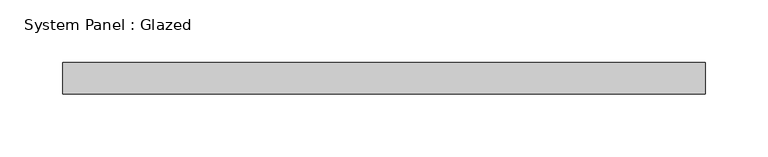
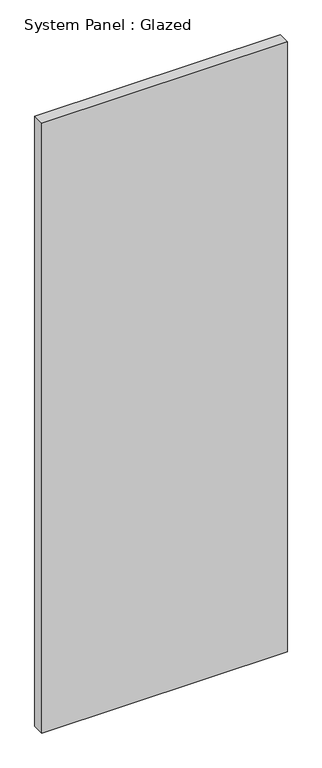
"""IFC4 building model written with IfcOpenShell, lengths in millimetres: plate geometry, System Panel : Glazed."""

from ifc_helpers import new_model, si_unit, origin, origin_with_axes, place, context, project, spatial, polyline, outline, extrude, source, transform, mapped, element, save


def system_panel_glazed_f9beff23(model_context):
    return source(origin(), model_context, "Body", "SweptSolid", [
        extrude(outline(polyline([(257.175, 19.05), (-257.175, 19.05), (-257.175, 44.45), (257.175, 44.45), (257.175, 19.05)])), origin_with_axes(), (0.0, 0.0, 1.0), 1350.1971055),
    ])


if __name__ == "__main__":
    model = new_model("IFC4")
    model_context = context("Model", 3, world=origin())
    ifc_project = project(units=[si_unit("LENGTHUNIT", "METRE", prefix="MILLI")], contexts=[model_context])
    site = spatial("IfcSite", under=ifc_project)
    building = spatial("IfcBuilding", under=site)
    placement = place(None, origin())
    system_panel_glazed_shape = system_panel_glazed_f9beff23(model_context)
    element("IfcPlate", 1, ObjectType="System Panel : Glazed", at=placement, inside=building, context=model_context, shape_type="MappedRepresentation", body=[
        mapped(system_panel_glazed_shape, transform((0.0, 0.0, 0.0), x_axis=(1.0, 0.0, 0.0), y_axis=(0.0, 1.0, 0.0), z_axis=(0.0, 0.0, 1.0))),
    ])
    save(model, "model.ifc")

# Revit data of these elements
# Type "System Panel : Glazed"
#   Construction Type Id = "GSP4R"
#   Analytic Construction = "1/8 in Pilkington single glazing"
#   Visual Light Transmittance = 0.9
#   Solar Heat Gain Coefficient = 0.86
#   Heat Transfer Coefficient (U) = 1.18115 BTU/(h·ft²·°F)
#   Define Thermal Properties by = 1
# Element 1 (IfcPlate, "System Panel : Glazed")
#   Materials on its faces: "Glass"
# Materials
#   "Glass": class "Glass", colour RGB 0 128 192, transparency 0.75, Description = "Soda Lime Glass", Cost = 0
